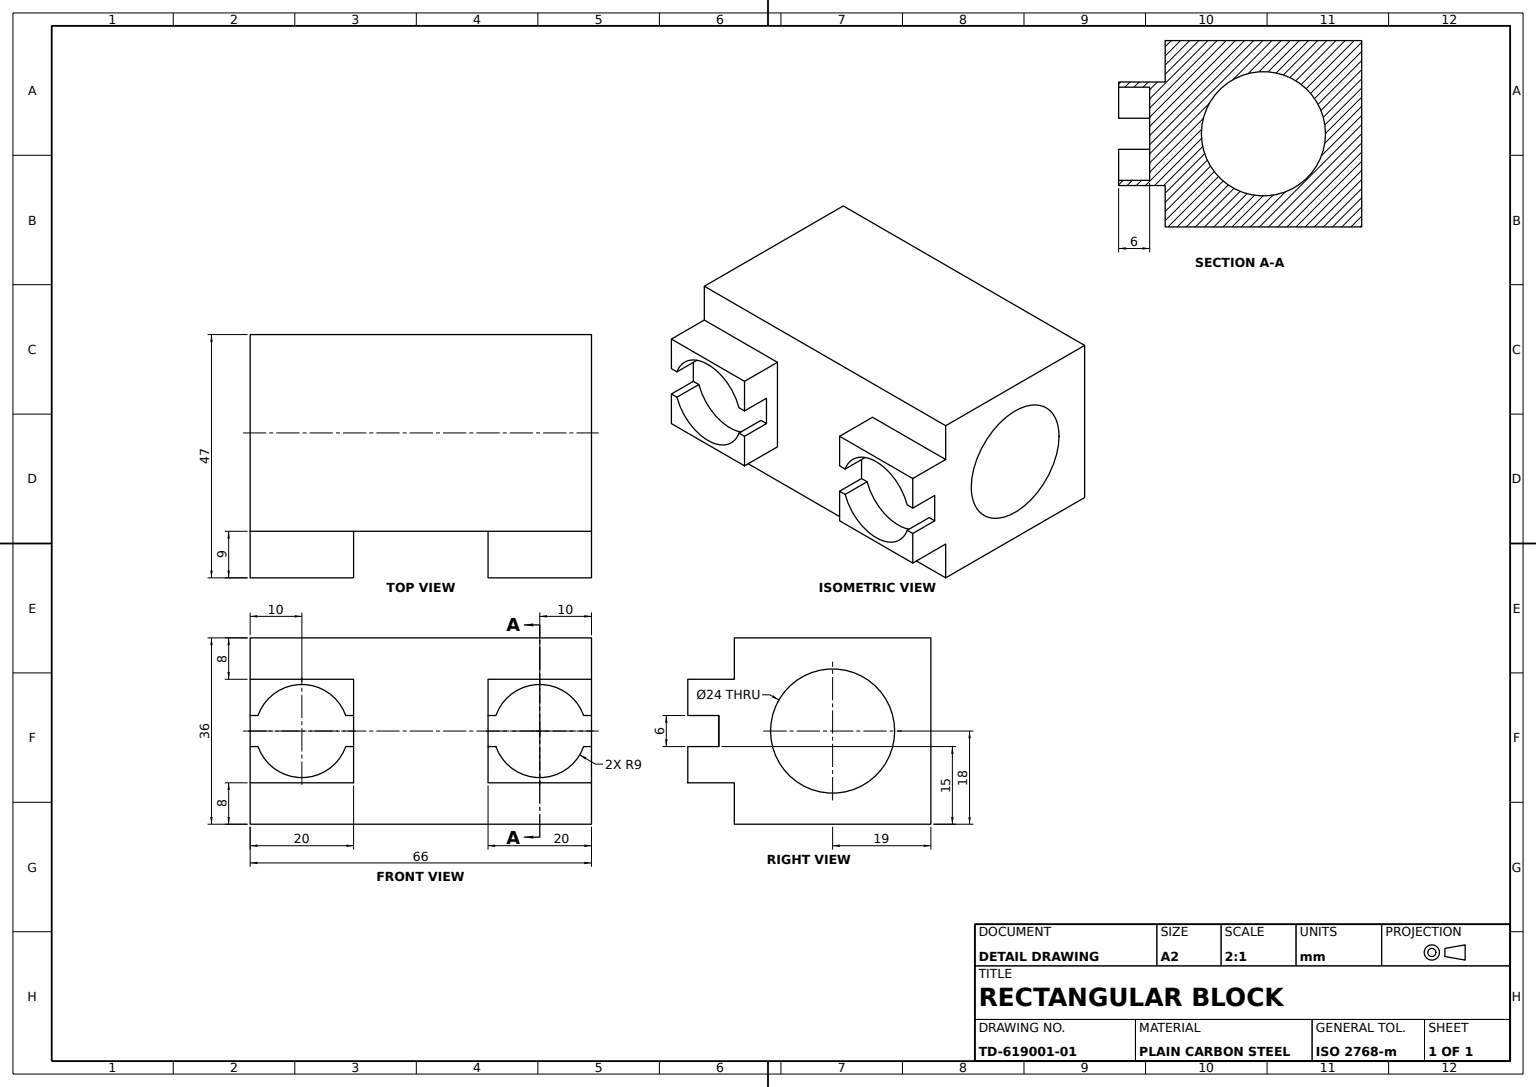
from build123d import *

# Parameters (mm, degrees)
MAIN_BLOCK_PROFILE_W      = 66
MAIN_BLOCK_PROFILE_H      = 36
MAIN_BLOCK_66X36X38_DEPTH = 38
CLAMP_BOSSES_PROFILE_W    = 20
CLAMP_BOSSES_PROFILE_H    = 20
CLAMP_BOSSES_DEPTH        = 9
SADDLE_CUT_18_A_PROFILE_R = 9
SADDLE_CUT_18_A_DEPTH     = 6
NOTCH_A_3X3_DEPTH         = 84
NOTCH_A_3X3_DEPTH_BACK    = 6
NOTCH_B_3X3_DEPTH         = 6
SADDLE_CUT_18_B_PROFILE_R = 9
SADDLE_CUT_18_B_DEPTH     = 6
NOTCH_C_3X3_DEPTH         = 6
NOTCH_D_PROFILE_W         = 6
NOTCH_D_PROFILE_H         = 6
NOTCH_D_DEPTH             = 6
END_BORE_24_PROFILE_R     = 12
END_BORE_24_DEPTH         = 84


with BuildPart() as part:
    # Main Block Profile → Main Block 66x36x38 (new body)
    with BuildSketch(Plane(origin=(0, 0, 0), x_dir=(0, 0, -1), z_dir=(1, 0, 0))):
        Rectangle(MAIN_BLOCK_PROFILE_W, MAIN_BLOCK_PROFILE_H)
    extrude(amount=MAIN_BLOCK_66X36X38_DEPTH)

    # Clamp Bosses Profile → Clamp Bosses (add)
    with BuildSketch(Plane(origin=(38, 0, 0), x_dir=(0, 0, -1), z_dir=(1, 0, 0))):
        with Locations((-23, 0)):
            Rectangle(CLAMP_BOSSES_PROFILE_W, CLAMP_BOSSES_PROFILE_H)
        with Locations((23, 0)):
            Rectangle(CLAMP_BOSSES_PROFILE_W, CLAMP_BOSSES_PROFILE_H)
    extrude(amount=CLAMP_BOSSES_DEPTH)

    # Saddle Cut Ø18 A Profile → Saddle Cut Ø18 A (cut)
    with BuildSketch(Plane(origin=(47, 0, 0), x_dir=(0, 0, -1), z_dir=(1, 0, 0))):
        with Locations((-23, 0)):
            Circle(SADDLE_CUT_18_A_PROFILE_R)
    extrude(amount=-SADDLE_CUT_18_A_DEPTH, mode=Mode.SUBTRACT)

    # Notch A Profile → Notch A 3x3 (cut, two sides: drawn at the far end of the back side and taken through both)
    with BuildSketch(Plane.XY.offset(33).offset(-NOTCH_A_3X3_DEPTH_BACK)):
        Polygon((41, 3), (41, 0), (41, -3), (47, -3), (47, 3), align=None)
    extrude(amount=NOTCH_A_3X3_DEPTH + NOTCH_A_3X3_DEPTH_BACK, mode=Mode.SUBTRACT)

    # Notch B Profile → Notch B 3x3 (cut)
    with BuildSketch(Plane(origin=(0, 0, 13), x_dir=(-1, 0, 0), z_dir=(0, 0, -1))):
        Polygon((-41, 0), (-41, 3), (-47, 3), (-47, -3), (-41, -3), align=None)
    extrude(amount=-NOTCH_B_3X3_DEPTH, mode=Mode.SUBTRACT)

    # Saddle Cut Ø18 B Profile → Saddle Cut Ø18 B (cut)
    with BuildSketch(Plane(origin=(47, 0, 0), x_dir=(0, 0, -1), z_dir=(1, 0, 0))):
        with Locations((23, 0)):
            Circle(SADDLE_CUT_18_B_PROFILE_R)
    extrude(amount=-SADDLE_CUT_18_B_DEPTH, mode=Mode.SUBTRACT)

    # Notch C Profile → Notch C 3x3 (cut)
    with BuildSketch(Plane(origin=(0, 0, -33), x_dir=(-1, 0, 0), z_dir=(0, 0, -1))):
        Polygon((-41, 0), (-41, 3), (-47, 3), (-47, -3), (-41, -3), align=None)
    extrude(amount=-NOTCH_C_3X3_DEPTH, mode=Mode.SUBTRACT)

    # Notch D Profile → Notch D (cut)
    with BuildSketch(Plane.XY.offset(-13)):
        with Locations((44, 0)):
            Rectangle(NOTCH_D_PROFILE_W, NOTCH_D_PROFILE_H)
    extrude(amount=-NOTCH_D_DEPTH, mode=Mode.SUBTRACT)

    # End Bore Ø24 Profile → End Bore Ø24 (cut, through all)
    with BuildSketch(Plane.XY.offset(33)):
        with Locations((19, 0)):
            Circle(END_BORE_24_PROFILE_R)
    extrude(amount=-END_BORE_24_DEPTH, mode=Mode.SUBTRACT)


solid = part.part
